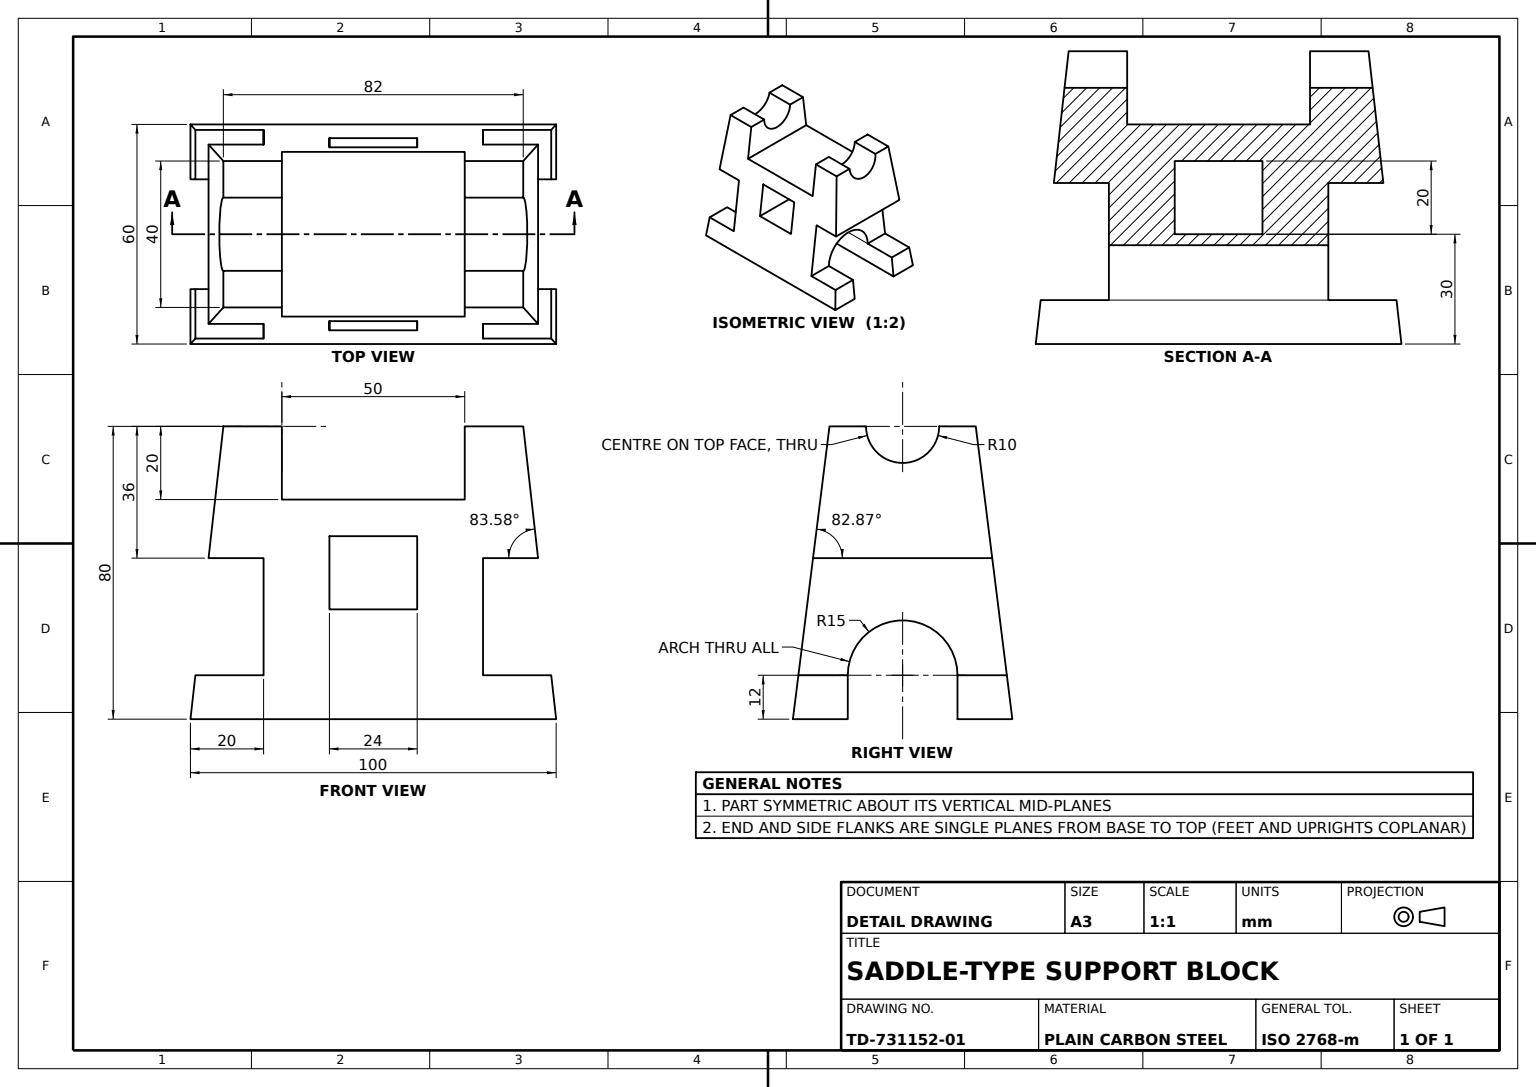
from build123d import *

# Parameters (mm, degrees)
FEET_AND_UPRIGHTS_CUT_DEPTH          = 99.994949528
FEET_AND_UPRIGHTS_CUT_DEPTH_BACK     = 99.994949528
FEET_AND_UPRIGHTS_PROFILE_SKETCH_W   = 29.409363616
FEET_AND_UPRIGHTS_PROFILE_SKETCH_H   = 32
FEET_AND_UPRIGHTS_PROFILE_SKETCH_W_2 = 50
FEET_AND_UPRIGHTS_PROFILE_SKETCH_H_2 = 20
BASE_ARCH_CUT_DEPTH                  = 99.994949528
BASE_ARCH_CUT_DEPTH_BACK             = 99.994949528
CRADLE_SADDLES_CUT_DEPTH             = 99.994949528
CRADLE_SADDLES_CUT_DEPTH_BACK        = 99.994949528
WEB_WINDOW_CUT_DEPTH                 = 99.994949528
WEB_WINDOW_CUT_DEPTH_BACK            = 99.994949528
WEB_WINDOW_SKETCH_W                  = 24
WEB_WINDOW_SKETCH_H                  = 20


with BuildPart() as part:
    # Base Profile Sketch → Tapered Block Loft section 0
    with BuildSketch(Plane(origin=(0, 0, 0), x_dir=(1, 0, 0), z_dir=(0, 1, 0))):
        with BuildLine():
            Line((-50, -30), (50, -30))
            Line((50, -30), (50, 30))
            Line((50, 30), (-50, 30))
            Line((-50, 30), (-50, -30))
        make_face()
    # Top Profile Sketch → Tapered Block Loft section 1
    with BuildSketch(Plane(origin=(0, 80, 0), x_dir=(1, 0, 0), z_dir=(0, 1, 0))):
        with BuildLine():
            Line((-41, -20), (41, -20))
            Line((41, -20), (41, 20))
            Line((41, 20), (-41, 20))
            Line((-41, 20), (-41, -20))
        make_face()
    loft()

    # Feet and Uprights Profile Sketch → Feet and Uprights Cut (cut, two sides: drawn at the far end of the back side and taken through both)
    with BuildSketch(Plane.XY.offset(-FEET_AND_UPRIGHTS_CUT_DEPTH_BACK)):
        with Locations((-44.704681808, 28)):
            Rectangle(FEET_AND_UPRIGHTS_PROFILE_SKETCH_W, FEET_AND_UPRIGHTS_PROFILE_SKETCH_H)
        with Locations((0, 70)):
            Rectangle(FEET_AND_UPRIGHTS_PROFILE_SKETCH_W_2, FEET_AND_UPRIGHTS_PROFILE_SKETCH_H_2)
        with Locations((44.704681808, 28)):
            Rectangle(FEET_AND_UPRIGHTS_PROFILE_SKETCH_W, FEET_AND_UPRIGHTS_PROFILE_SKETCH_H)
    extrude(amount=FEET_AND_UPRIGHTS_CUT_DEPTH + FEET_AND_UPRIGHTS_CUT_DEPTH_BACK, mode=Mode.SUBTRACT)

    # Base Arch Sketch → Base Arch Cut (cut, two sides: drawn at the far end of the back side and taken through both)
    with BuildSketch(Plane(origin=(0, 0, 0), x_dir=(0, 0, -1), z_dir=(1, 0, 0)).offset(-BASE_ARCH_CUT_DEPTH_BACK)):
        with BuildLine():
            Line((-10, 80), (10, 80))
            ThreePointArc((10, 80), (0, 70), (-10, 80))
        make_face()
    extrude(amount=BASE_ARCH_CUT_DEPTH + BASE_ARCH_CUT_DEPTH_BACK, mode=Mode.SUBTRACT)

    # Cradle Saddles Sketch → Cradle Saddles Cut (cut, two sides: drawn at the far end of the back side and taken through both)
    with BuildSketch(Plane(origin=(0, 0, 0), x_dir=(0, 0, -1), z_dir=(1, 0, 0)).offset(-CRADLE_SADDLES_CUT_DEPTH_BACK)):
        with BuildLine():
            Line((-15, 12), (-15, 0))
            Line((-15, 0), (15, 0))
            Line((15, 0), (15, 12))
            ThreePointArc((15, 12), (0, 27), (-15, 12))
        make_face()
    extrude(amount=CRADLE_SADDLES_CUT_DEPTH + CRADLE_SADDLES_CUT_DEPTH_BACK, mode=Mode.SUBTRACT)

    # Web Window Sketch → Web Window Cut (cut, two sides: drawn at the far end of the back side and taken through both)
    with BuildSketch(Plane.XY.offset(-WEB_WINDOW_CUT_DEPTH_BACK)):
        with Locations((0, 40)):
            Rectangle(WEB_WINDOW_SKETCH_W, WEB_WINDOW_SKETCH_H)
    extrude(amount=WEB_WINDOW_CUT_DEPTH + WEB_WINDOW_CUT_DEPTH_BACK, mode=Mode.SUBTRACT)


solid = part.part
